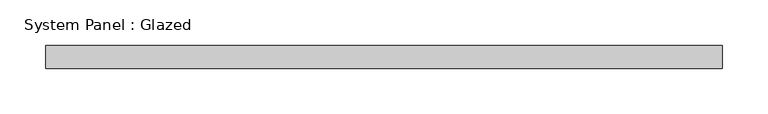
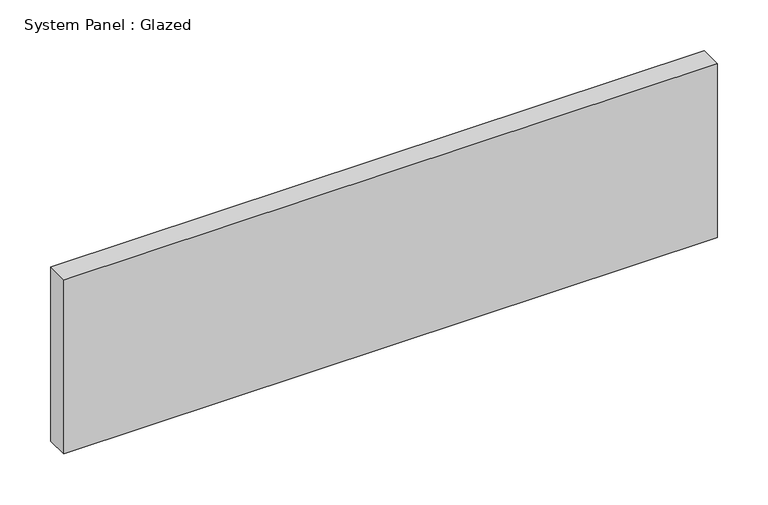
"""IFC4 building model written with IfcOpenShell, lengths in millimetres: plate geometry, System Panel : Glazed."""

from ifc_helpers import new_model, si_unit, origin, origin_with_axes, place, context, project, spatial, polyline, outline, extrude, source, transform, mapped, element, save


def system_panel_glazed_2bc0fbab(model_context):
    return source(origin(), model_context, "Body", "SweptSolid", [
        extrude(outline(polyline([(371.475, 19.05), (-371.475, 19.05), (-371.475, 44.45), (371.475, 44.45), (371.475, 19.05)])), origin_with_axes(), (0.0, 0.0, 1.0), 209.55),
    ])


if __name__ == "__main__":
    model = new_model("IFC4")
    model_context = context("Model", 3, world=origin())
    ifc_project = project(units=[si_unit("LENGTHUNIT", "METRE", prefix="MILLI")], contexts=[model_context])
    site = spatial("IfcSite", under=ifc_project)
    building = spatial("IfcBuilding", under=site)
    placement = place(None, origin())
    system_panel_glazed_shape = system_panel_glazed_2bc0fbab(model_context)
    element("IfcPlate", 1, ObjectType="System Panel : Glazed", at=placement, inside=building, context=model_context, shape_type="MappedRepresentation", body=[
        mapped(system_panel_glazed_shape, transform((0.0, 0.0, 0.0), x_axis=(1.0, 0.0, 0.0), y_axis=(0.0, 1.0, 0.0), z_axis=(0.0, 0.0, 1.0))),
    ])
    save(model, "model.ifc")

# Revit data of these elements
# Type "System Panel : Glazed"
#   Construction Type Id = "GSP4R"
#   Analytic Construction = "1/8 in Pilkington single glazing"
#   Visual Light Transmittance = 0.9
#   Solar Heat Gain Coefficient = 0.86
#   Heat Transfer Coefficient (U) = 1.18115 BTU/(h·ft²·°F)
#   Define Thermal Properties by = 1
# Element 1 (IfcPlate, "System Panel : Glazed")
#   Materials on its faces: "Glass"
# Materials
#   "Glass": class "Glass", colour RGB 0 128 192, transparency 0.75, Description = "Soda Lime Glass", Cost = 0
